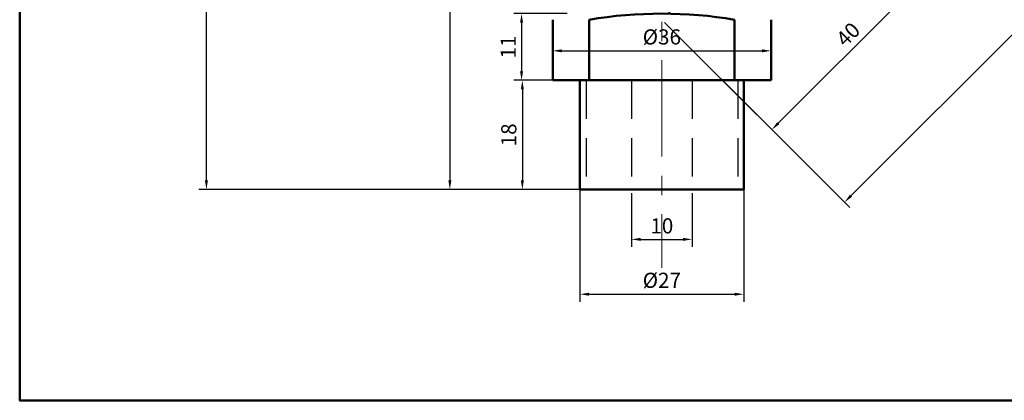
# Model space of a CAD drawing. Units: millimetres. Extents: x -414 to 17, y 81 to 417.
# Tile 1 of 7: x -414 to -252, y 81 to 143. Entities that reach past the tile are written whole.
import ezdxf

# ---------------------------------------------------------------- set-up
doc = ezdxf.new("R2010")
doc.units = ezdxf.units.MM
doc.header["$LTSCALE"] = 0.5
doc.linetypes.add('CENTER', pattern=[50.8, 31.75, -6.35, 6.35, -6.35])
doc.linetypes.add('DASHED', pattern=[19.05, 12.7, -6.35])
for name, color, linetype, lineweight in [('M-CNTR', 1, 'CENTER', 18), ('M-DIMS', 2, 'Continuous', 25), ('M-HIDN', 6, 'DASHED', 25), ('M-OUTL', 7, 'Continuous', 50)]:
    doc.layers.add(name, color=color, linetype=linetype, lineweight=lineweight)
doc.styles.get("Standard").update_dxf_attribs({"font": 'arial.ttf'})
doc.dimstyles.new('ISO-25', dxfattribs={"dimtxt": 2.5, "dimasz": 1.5, "dimexe": 1.25, "dimexo": 0.625, "dimtad": 1, "dimtoh": 1, "dimdec": 0, "dimtxsty": 'Standard', "dimcen": 2.5, "dimadec": 0, "dimazin": 0, "dimtfac": 1, "dimtdec": 0, "dimtmove": 0, "dimatfit": 3, "dimfxl": 1, "dimarcsym": 0})

# ---------------------------------------------------------------- blocks, each defined once
blk = doc.blocks.new('*D41')
at = {"layer": 'Defpoints', "color": 0, "ltscale": 0.5, "transparency": 16777216}
for p in [(-383.58, 200.46), (-351.8, 200.46), (-308.49, 115.46)]:
    blk.add_point(p, dxfattribs=at)
at = {"layer": 'M-DIMS', "color": 0, "lineweight": -2, "ltscale": 0.5, "transparency": 16777216}
for p, q in [((-352.42, 200.46), (-384.83, 200.46)), ((-383.58, 116.96), (-383.58, 198.96)), ((-309.12, 115.46), (-384.83, 115.46))]:
    blk.add_line(p, q, dxfattribs=at)
at = {"layer": 'M-DIMS', "color": 0, "ltscale": 0.5, "transparency": 16777216}
for points in [[(-383.83, 198.96), (-383.33, 198.96), (-383.58, 200.46)], [(-383.83, 116.96), (-383.33, 116.96), (-383.58, 115.46)]]:
    blk.add_solid(points, dxfattribs=at)
at = {"layer": 'M-DIMS', "color": 0, "ltscale": 0.5, "transparency": 16777216, "insert": (-385.48, 157.96), "char_height": 2.5, "attachment_point": 5, "rotation": 90}
blk.add_mtext('85', dxfattribs=at)
blk = doc.blocks.new('*D42')
at = {"layer": 'Defpoints', "color": 0, "ltscale": 0.5, "transparency": 16777216}
for p in [(-313.49, 115.46), (-303.49, 115.46), (-303.49, 107.22)]:
    blk.add_point(p, dxfattribs=at)
at = {"layer": 'M-DIMS', "color": 0, "lineweight": -2, "ltscale": 0.5, "transparency": 16777216}
for p, q in [((-313.49, 114.84), (-313.49, 105.97)), ((-303.49, 114.84), (-303.49, 105.97)), ((-311.99, 107.22), (-304.99, 107.22))]:
    blk.add_line(p, q, dxfattribs=at)
at = {"layer": 'M-DIMS', "color": 0, "ltscale": 0.5, "transparency": 16777216}
for points in [[(-311.99, 107.47), (-311.99, 106.97), (-313.49, 107.22)], [(-304.99, 107.47), (-304.99, 106.97), (-303.49, 107.22)]]:
    blk.add_solid(points, dxfattribs=at)
at = {"layer": 'M-DIMS', "color": 0, "ltscale": 0.5, "transparency": 16777216, "insert": (-308.49, 109.12), "char_height": 2.5, "attachment_point": 5}
blk.add_mtext('10', dxfattribs=at)
blk = doc.blocks.new('*D43')
at = {"layer": 'Defpoints', "color": 0, "ltscale": 0.5, "transparency": 16777216}
for p in [(-321.99, 128.53), (-294.99, 128.53), (-294.99, 98.17)]:
    blk.add_point(p, dxfattribs=at)
at = {"layer": 'M-DIMS', "color": 0, "lineweight": -2, "ltscale": 0.5, "transparency": 16777216}
for p, q in [((-321.99, 127.91), (-321.99, 96.92)), ((-294.99, 127.91), (-294.99, 96.92)), ((-320.49, 98.17), (-296.49, 98.17))]:
    blk.add_line(p, q, dxfattribs=at)
at = {"layer": 'M-DIMS', "color": 0, "ltscale": 0.5, "transparency": 16777216}
for points in [[(-320.49, 98.42), (-320.49, 97.92), (-321.99, 98.17)], [(-296.49, 98.42), (-296.49, 97.92), (-294.99, 98.17)]]:
    blk.add_solid(points, dxfattribs=at)
at = {"layer": 'M-DIMS', "color": 0, "ltscale": 0.5, "transparency": 16777216, "insert": (-308.49, 100.14), "char_height": 2.5, "attachment_point": 5}
blk.add_mtext('%%C27', dxfattribs=at)
blk = doc.blocks.new('*D45')
at = {"layer": 'Defpoints', "color": 0, "ltscale": 0.5, "transparency": 16777216}
for p in [(-342.26, 180.96), (-343.44, 115.46), (-342.26, 115.46)]:
    blk.add_point(p, dxfattribs=at)
at = {"layer": 'M-DIMS', "color": 0, "lineweight": -2, "ltscale": 0.5, "transparency": 16777216}
for p, q in [((-342.88, 180.96), (-344.69, 180.96)), ((-343.44, 179.46), (-343.44, 116.96)), ((-342.88, 115.46), (-344.69, 115.46))]:
    blk.add_line(p, q, dxfattribs=at)
at = {"layer": 'M-DIMS', "color": 0, "ltscale": 0.5, "transparency": 16777216}
for points in [[(-343.69, 179.46), (-343.19, 179.46), (-343.44, 180.96)], [(-343.69, 116.96), (-343.19, 116.96), (-343.44, 115.46)]]:
    blk.add_solid(points, dxfattribs=at)
at = {"layer": 'M-DIMS', "color": 0, "ltscale": 0.5, "transparency": 16777216, "insert": (-345.34, 148.21), "char_height": 2.5, "attachment_point": 5, "rotation": 90}
blk.add_mtext('66', dxfattribs=at)
blk = doc.blocks.new('*D46')
at = {"layer": 'Defpoints', "color": 0, "ltscale": 0.5, "transparency": 16777216}
for p in [(-326.49, 133.46), (-331.49, 115.46), (-326.49, 115.46)]:
    blk.add_point(p, dxfattribs=at)
at = {"layer": 'M-DIMS', "color": 0, "lineweight": -2, "ltscale": 0.5, "transparency": 16777216}
for p, q in [((-327.12, 133.46), (-332.74, 133.46)), ((-331.49, 131.96), (-331.49, 116.96)), ((-327.12, 115.46), (-332.74, 115.46))]:
    blk.add_line(p, q, dxfattribs=at)
at = {"layer": 'M-DIMS', "color": 0, "ltscale": 0.5, "transparency": 16777216}
for points in [[(-331.74, 131.96), (-331.24, 131.96), (-331.49, 133.46)], [(-331.74, 116.96), (-331.24, 116.96), (-331.49, 115.46)]]:
    blk.add_solid(points, dxfattribs=at)
at = {"layer": 'M-DIMS', "color": 0, "ltscale": 0.5, "transparency": 16777216, "insert": (-333.4, 124.46), "char_height": 2.5, "attachment_point": 5, "rotation": 90}
blk.add_mtext('18', dxfattribs=at)
blk = doc.blocks.new('*D47')
at = {"layer": 'Defpoints', "color": 0, "ltscale": 0.5, "transparency": 16777216}
for p in [(-323.49, 144.46), (-331.62, 133.46), (-323.49, 133.46)]:
    blk.add_point(p, dxfattribs=at)
at = {"layer": 'M-DIMS', "color": 0, "lineweight": -2, "ltscale": 0.5, "transparency": 16777216}
for p, q in [((-324.12, 144.46), (-332.87, 144.46)), ((-331.62, 142.96), (-331.62, 134.96)), ((-324.12, 133.46), (-332.87, 133.46))]:
    blk.add_line(p, q, dxfattribs=at)
at = {"layer": 'M-DIMS', "color": 0, "ltscale": 0.5, "transparency": 16777216}
for points in [[(-331.87, 142.96), (-331.37, 142.96), (-331.62, 144.46)], [(-331.87, 134.96), (-331.37, 134.96), (-331.62, 133.46)]]:
    blk.add_solid(points, dxfattribs=at)
at = {"layer": 'M-DIMS', "color": 0, "ltscale": 0.5, "transparency": 16777216, "insert": (-333.5, 138.96), "char_height": 2.5, "attachment_point": 5, "rotation": 90}
blk.add_mtext('11', dxfattribs=at)
blk = doc.blocks.new('*D48')
at = {"layer": 'Defpoints', "color": 0, "ltscale": 0.5, "transparency": 16777216}
for p in [(-290.49, 138.32), (-326.49, 136.43), (-290.49, 136.43)]:
    blk.add_point(p, dxfattribs=at)
at = {"layer": 'M-DIMS', "color": 0, "lineweight": -2, "ltscale": 0.5, "transparency": 16777216}
for p, q in [((-326.49, 137.05), (-326.49, 139.57)), ((-324.99, 138.32), (-291.99, 138.32)), ((-290.49, 137.05), (-290.49, 139.57))]:
    blk.add_line(p, q, dxfattribs=at)
at = {"layer": 'M-DIMS', "color": 0, "ltscale": 0.5, "transparency": 16777216}
for points in [[(-324.99, 138.57), (-324.99, 138.07), (-326.49, 138.32)], [(-291.99, 138.57), (-291.99, 138.07), (-290.49, 138.32)]]:
    blk.add_solid(points, dxfattribs=at)
at = {"layer": 'M-DIMS', "color": 0, "ltscale": 0.5, "transparency": 16777216, "insert": (-308.49, 140.29), "char_height": 2.5, "attachment_point": 5}
blk.add_mtext('%%C36', dxfattribs=at)
blk = doc.blocks.new('*D69')
at = {"layer": 'Defpoints', "color": 0, "ltscale": 0.5, "transparency": 16777216}
for p in [(-280.21, 171.75), (-262.07, 153.61), (-308.49, 143.46)]:
    blk.add_point(p, dxfattribs=at)
at = {"layer": 'M-DIMS', "color": 0, "lineweight": -2, "ltscale": 0.5, "transparency": 16777216}
for p, q in [((-279.77, 171.3), (-261.19, 152.72)), ((-289.29, 126.38), (-263.13, 152.55)), ((-308.05, 143.02), (-289.47, 124.44))]:
    blk.add_line(p, q, dxfattribs=at)
at = {"layer": 'M-DIMS', "color": 0, "ltscale": 0.5, "transparency": 16777216}
for points in [[(-263.31, 152.72), (-262.95, 152.37), (-262.07, 153.61)], [(-289.47, 126.56), (-289.12, 126.21), (-290.35, 125.32)]]:
    blk.add_solid(points, dxfattribs=at)
at = {"layer": 'M-DIMS', "color": 0, "ltscale": 0.5, "transparency": 16777216, "insert": (-277.56, 140.81), "char_height": 2.5, "attachment_point": 5, "rotation": 45}
blk.add_mtext('40', dxfattribs=at)
blk = doc.blocks.new('*D70')
at = {"layer": 'Defpoints', "color": 0, "ltscale": 0.5, "transparency": 16777216}
for p in [(-222.23, 229.73), (-308.49, 143.46), (-278.37, 113.34)]:
    blk.add_point(p, dxfattribs=at)
at = {"layer": 'M-DIMS', "color": 0, "lineweight": -2, "ltscale": 0.5, "transparency": 16777216}
for p, q in [((-221.78, 229.29), (-191.22, 198.73)), ((-193.17, 198.55), (-277.31, 114.4)), ((-308.05, 143.02), (-277.49, 112.46))]:
    blk.add_line(p, q, dxfattribs=at)
at = {"layer": 'M-DIMS', "color": 0, "ltscale": 0.5, "transparency": 16777216}
for points in [[(-193.34, 198.73), (-192.99, 198.37), (-192.11, 199.61)], [(-277.49, 114.58), (-277.14, 114.23), (-278.37, 113.34)]]:
    blk.add_solid(points, dxfattribs=at)
at = {"layer": 'M-DIMS', "color": 0, "ltscale": 0.5, "transparency": 16777216, "insert": (-236.57, 157.81), "char_height": 2.5, "attachment_point": 5, "rotation": 45}
blk.add_mtext('122', dxfattribs=at)
blk = doc.blocks.new('*D78')
at = {"layer": 'Defpoints', "color": 0, "ltscale": 0.5, "transparency": 16777216}
for p in [(-308.49, 365.43), (-250.63, 243.68), (-212.22, 239.73), (-308.49, 230.96), (-308.49, 143.46)]:
    blk.add_point(p, dxfattribs=at)
at = {"layer": 'M-DIMS', "color": 0, "lineweight": -2, "ltscale": 0.5, "transparency": 16777216}
blk.add_arc((-308.49, 143.46), 115.73, 45.7426, 89.2574, dxfattribs=at)
at = {"layer": 'M-DIMS', "color": 0, "ltscale": 0.5, "transparency": 16777216}
for points in [[(-306.99, 258.93), (-306.99, 259.43), (-308.49, 259.19)], [(-227.55, 226.52), (-227.9, 226.17), (-226.66, 225.29)]]:
    blk.add_solid(points, dxfattribs=at)
at = {"layer": 'M-DIMS', "color": 0, "ltscale": 0.5, "transparency": 16777216, "insert": (-263.48, 252.13), "char_height": 2.5, "attachment_point": 5, "rotation": 337.5}
blk.add_mtext('45°', dxfattribs=at)

msp = doc.modelspace()

# ---------------------------------------------------------------- linework, layer by layer
at = {"layer": 'M-CNTR', "ltscale": 0.5}
msp.add_line((-212.22, 239.73), (-308.49, 143.46), dxfattribs=at)
at = {"layer": 'M-CNTR'}
msp.add_line((-308.49, 212.96), (-308.49, 102.53), dxfattribs=at)
at = {"layer": 'M-HIDN'}
for p, q in [((-320.99, 133.46), (-320.99, 115.46)), ((-313.49, 133.46), (-313.49, 115.46)), ((-303.49, 133.46), (-303.49, 115.46)), ((-295.99, 133.46), (-295.99, 115.46))]:
    msp.add_line(p, q, dxfattribs=at)
at = {"layer": 'M-OUTL'}
for p, q in [((-326.49, 143.46), (-326.49, 133.46)), ((-320.49, 143.46), (-320.49, 133.46)), ((-296.49, 143.46), (-296.49, 133.46)), ((-290.49, 143.46), (-290.49, 133.46)), ((-321.99, 133.46), (-321.99, 115.46)), ((-294.99, 133.46), (-294.99, 115.46))]:
    msp.add_line(p, q, dxfattribs=at)
at = {"layer": 'M-OUTL', "ltscale": 0.5}
for p, q in [((-326.49, 133.46), (-290.49, 133.46)), ((-321.99, 115.46), (-294.99, 115.46))]:
    msp.add_line(p, q, dxfattribs=at)
msp.add_lwpolyline([(-414.36, 417.09), (16.87, 417.09), (16.87, 80.66), (-414.36, 80.66)], close=True, dxfattribs=at)
for centre, radius, start, end in [((-308.49, 71.96), 72.5, 80.4727, 99.5273), ((-289.61, 143.43), 0.879, 178.0179, 181.9821)]:
    msp.add_arc(centre, radius, start, end, dxfattribs=at)

# ---------------------------------------------------------------- dimensions: what is measured, and where the dimension line sits
at = {"layer": 'M-DIMS', "ltscale": 0.5}
dim = msp.add_angular_dim_2l(base=(-250.63, 243.68), line1=((-308.49, 365.43), (-308.49, 230.96)), line2=((-212.22, 239.73), (-308.49, 143.46)), dimstyle='ISO-25', override={"dimclrd": 0, "dimclre": 0, "dimclrt": 0}, dxfattribs=at)
dim.commit()
dim.dimension.update_dxf_attribs({"geometry": '*D78', "text_midpoint": (-263.48, 252.13)})
for p1, p2, distance, picture, middle in [((-222.23, 229.73), (-308.49, 143.46), 42.59, '*D70', (-236.57, 157.81)), ((-308.49, 143.46), (-280.21, 171.75), -25.65, '*D69', (-277.56, 140.81))]:
    dim = msp.add_aligned_dim(p1=p1, p2=p2, distance=distance, dimstyle='ISO-25', override={"dimclrd": 0, "dimclre": 0, "dimclrt": 0}, dxfattribs=at)
    dim.commit()
    dim.dimension.update_dxf_attribs({"geometry": picture, "text_midpoint": middle})
for base, p1, p2, picture, middle in [((-383.58, 200.46), (-308.49, 115.46), (-351.8, 200.46), '*D41', (-385.48, 157.96)), ((-343.43816969, 115.46126483), (-342.25706478, 180.96126483), (-342.25706478, 115.46126483), '*D45', (-345.33960216, 148.21126483)), ((-331.62, 133.46), (-323.49, 144.46), (-323.49, 133.46), '*D47', (-333.5, 138.96)), ((-331.49, 115.46), (-326.49, 133.46), (-326.49, 115.46), '*D46', (-333.4, 124.46))]:
    dim = msp.add_linear_dim(base=base, p1=p1, p2=p2, angle=90, dimstyle='ISO-25', override={"dimclrd": 0, "dimclre": 0, "dimclrt": 0}, dxfattribs=at)
    dim.commit()
    dim.dimension.update_dxf_attribs({"geometry": picture, "text_midpoint": middle})
for base, p1, p2, picture, middle in [((-290.49, 138.32), (-326.49, 136.43), (-290.49, 136.43), '*D48', (-308.49, 140.29)), ((-294.99, 98.17), (-321.99, 128.53), (-294.99, 128.53), '*D43', (-308.49, 100.14))]:
    dim = msp.add_linear_dim(base=base, p1=p1, p2=p2, text='%%C<>', dimstyle='ISO-25', override={"dimclrd": 0, "dimclre": 0, "dimclrt": 0}, dxfattribs=at)
    dim.commit()
    dim.dimension.update_dxf_attribs({"geometry": picture, "text_midpoint": middle})
dim = msp.add_linear_dim(base=(-303.49, 107.22), p1=(-313.49, 115.46), p2=(-303.49, 115.46), dimstyle='ISO-25', override={"dimclrd": 0, "dimclre": 0, "dimclrt": 0}, dxfattribs=at)
dim.commit()
dim.dimension.update_dxf_attribs({"geometry": '*D42', "text_midpoint": (-308.49, 109.12)})

doc.saveas('drawing.dxf')
